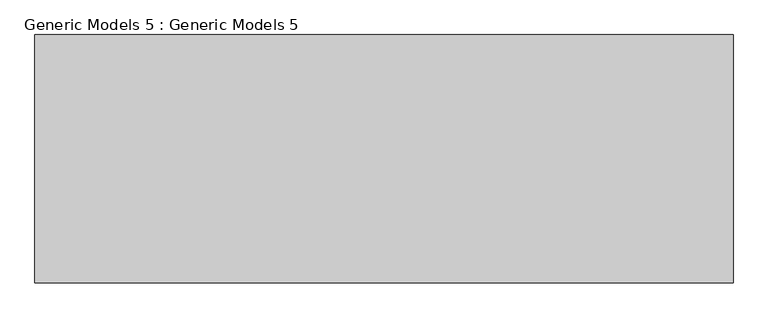
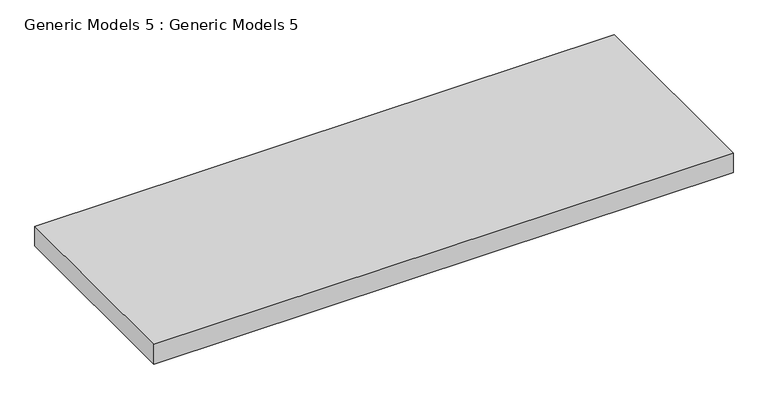
"""IFC4 building model written with IfcOpenShell, lengths in millimetres: proxy geometry, Generic Models 5 : Generic Models 5."""

from ifc_helpers import new_model, si_unit, frame, origin, place, context, project, spatial, polyline, outline, extrude, source, transform, mapped, element, save


def generic_models_5_generic_models_5_d5554940(model_context):
    return source(origin(), model_context, "Body", "SweptSolid", [
        extrude(outline(polyline([(2856.4546869, -6539.1901953), (-3518.9453131, -6539.1901953), (-3518.9453131, -4272.2938352), (2856.4546869, -4272.2938352), (2856.4546869, -6539.1901953)])), frame((0.0, 0.0, 6400.8), z_axis=(0.0, 0.0, 1.0), x_axis=(1.0, 0.0, 0.0)), (0.0, 0.0, 1.0), 228.6),
    ])


if __name__ == "__main__":
    model = new_model("IFC4")
    model_context = context("Model", 3, world=origin())
    ifc_project = project(units=[si_unit("LENGTHUNIT", "METRE", prefix="MILLI")], contexts=[model_context])
    site = spatial("IfcSite", under=ifc_project)
    building = spatial("IfcBuilding", under=site)
    placement = place(None, origin())
    generic_models_5_generic_models_5_shape = generic_models_5_generic_models_5_d5554940(model_context)
    element("IfcBuildingElementProxy", 1, Name="Generic Models 5 : Generic Models 5", ObjectType="Generic Models 5 : Generic Models 5", at=placement, inside=building, context=model_context, shape_type="MappedRepresentation", body=[
        mapped(generic_models_5_generic_models_5_shape, transform((0.0, 0.0, 0.0), x_axis=(1.0, 0.0, 0.0), y_axis=(0.0, 1.0, 0.0), z_axis=(0.0, 0.0, 1.0))),
    ])
    save(model, "model.ifc")

# Revit data of these elements
# Element 1 (IfcBuildingElementProxy, "Generic Models 5 : Generic Models 5")
#   Materials on its faces: "WALL PAINT"
# Materials
#   "WALL PAINT": class "Generic", colour RGB 120 120 120, transparency 0, Cost = 0
